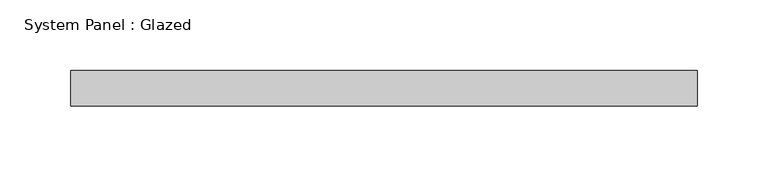
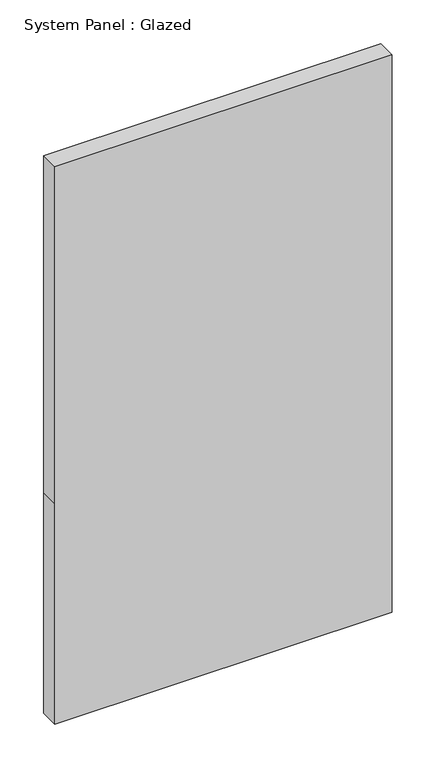
"""IFC4 building model written with IfcOpenShell, lengths in millimetres: plate geometry, System Panel : Glazed."""

from ifc_helpers import new_model, si_unit, frame, origin, place, context, project, spatial, polyline, outline, extrude, source, transform, mapped, element, save


def system_panel_glazed_af2b4658(model_context):
    return source(origin(), model_context, "Body", "SweptSolid", [
        extrude(outline(polyline([(0.0, -222.25), (0.0, 222.25), (306.9166667, 222.25), (776.8166667, 222.25), (776.8166667, -222.25), (306.9166667, -222.25), (0.0, -222.25)])), frame((0.0, 19.05, 0.0), z_axis=(0.0, 1.0, 0.0), x_axis=(0.0, 0.0, 1.0)), (0.0, 0.0, 1.0), 25.4),
    ])


if __name__ == "__main__":
    model = new_model("IFC4")
    model_context = context("Model", 3, world=origin())
    ifc_project = project(units=[si_unit("LENGTHUNIT", "METRE", prefix="MILLI")], contexts=[model_context])
    site = spatial("IfcSite", under=ifc_project)
    building = spatial("IfcBuilding", under=site)
    placement = place(None, origin())
    system_panel_glazed_shape = system_panel_glazed_af2b4658(model_context)
    element("IfcPlate", 1, ObjectType="System Panel : Glazed", at=placement, inside=building, context=model_context, shape_type="MappedRepresentation", body=[
        mapped(system_panel_glazed_shape, transform((0.0, 0.0, 0.0), x_axis=(1.0, 0.0, 0.0), y_axis=(0.0, 1.0, 0.0), z_axis=(0.0, 0.0, 1.0))),
    ])
    save(model, "model.ifc")

# Revit data of these elements
# Type "System Panel : Glazed"
#   Construction Type Id = "GSP4R"
#   Analytic Construction = "1/8 in Pilkington single glazing"
#   Visual Light Transmittance = 0.9
#   Solar Heat Gain Coefficient = 0.86
#   Heat Transfer Coefficient (U) = 1.18115 BTU/(h·ft²·°F)
#   Define Thermal Properties by = 1
# Element 1 (IfcPlate, "System Panel : Glazed")
#   Materials on its faces: "Glass"
# Materials
#   "Glass": class "Glass", colour RGB 0 128 192, transparency 0.75, Description = "Soda Lime Glass", Cost = 0
